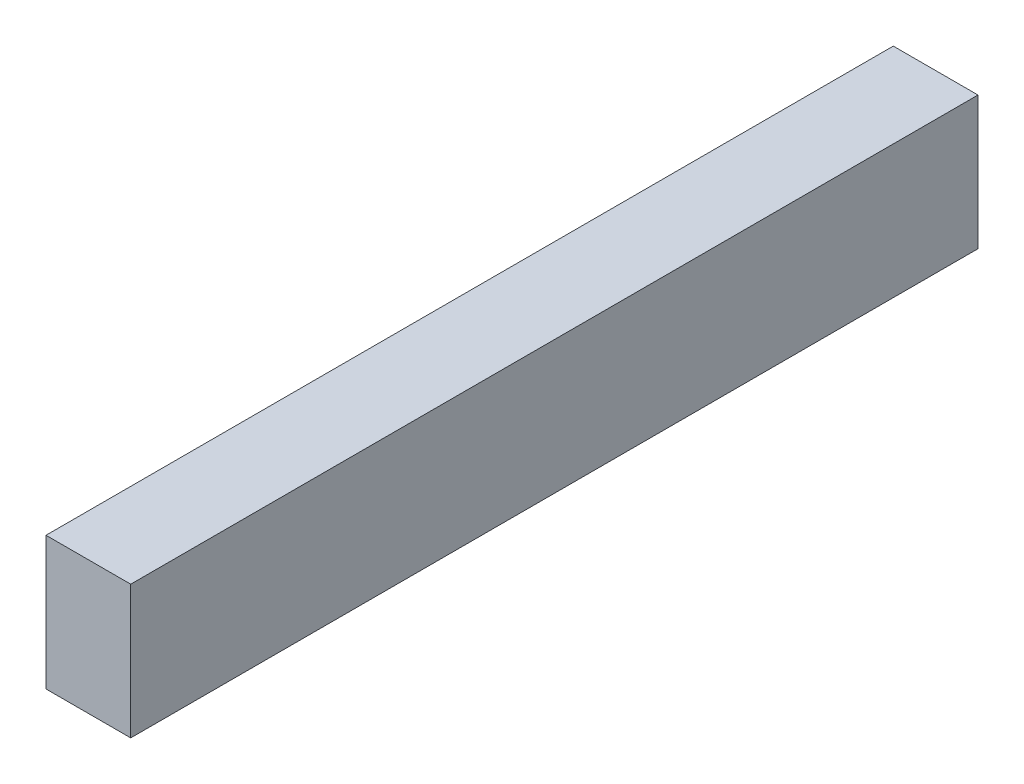
from build123d import *

# Parameters (mm, degrees)
KEY_SECTION_22X14_SKETCH_W = 14
KEY_SECTION_22X14_SKETCH_H = 22
KEY_BODY_140MM_DEPTH       = 70


with BuildPart() as part:
    # Key Section 22x14 Sketch → Key Body 140mm (new, symmetric)
    with BuildSketch(Plane.XY):
        Rectangle(KEY_SECTION_22X14_SKETCH_W, KEY_SECTION_22X14_SKETCH_H)
    extrude(amount=KEY_BODY_140MM_DEPTH, both=True)


solid = part.part
